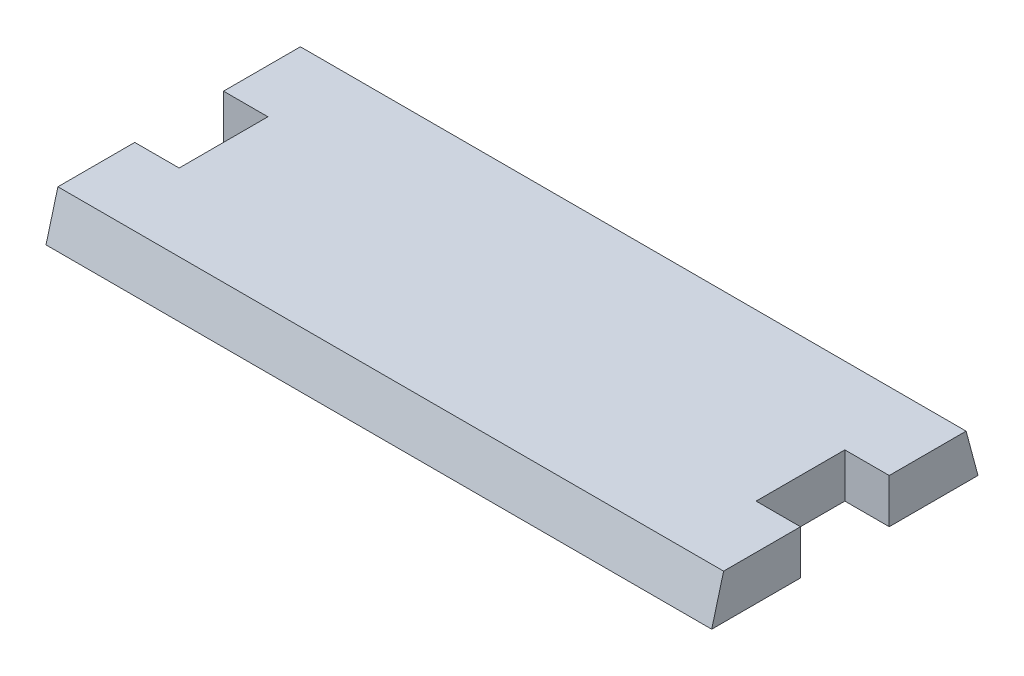
ISO-10303-21;
HEADER;
FILE_DESCRIPTION(('STEP AP214'),'2;1');
FILE_NAME('part.step','',(''),(''),'','','');
FILE_SCHEMA(('AUTOMOTIVE_DESIGN { 1 0 10303 214 1 1 1 1 }'));
ENDSEC;
DATA;
#1=APPLICATION_CONTEXT('core data for automotive mechanical design processes');
#2=APPLICATION_PROTOCOL_DEFINITION('international standard','automotive_design',2000,#1);
#3=PRODUCT_CONTEXT('',#1,'mechanical');
#4=PRODUCT('Part','Part','',(#3));
#5=PRODUCT_RELATED_PRODUCT_CATEGORY('part','',(#4));
#6=PRODUCT_DEFINITION_FORMATION('','',#4);
#7=PRODUCT_DEFINITION_CONTEXT('part definition',#1,'design');
#8=PRODUCT_DEFINITION('design','',#6,#7);
#9=PRODUCT_DEFINITION_SHAPE('','',#8);
#10=(LENGTH_UNIT() NAMED_UNIT(*) SI_UNIT(.MILLI.,.METRE.));
#11=(NAMED_UNIT(*) PLANE_ANGLE_UNIT() SI_UNIT($,.RADIAN.));
#12=(NAMED_UNIT(*) SI_UNIT($,.STERADIAN.) SOLID_ANGLE_UNIT());
#13=UNCERTAINTY_MEASURE_WITH_UNIT(LENGTH_MEASURE(1.E-05),#10,'distance_accuracy_value','');
#14=(GEOMETRIC_REPRESENTATION_CONTEXT(3) GLOBAL_UNCERTAINTY_ASSIGNED_CONTEXT((#13)) GLOBAL_UNIT_ASSIGNED_CONTEXT((#10,
#11,#12)) REPRESENTATION_CONTEXT('',''));
#15=CARTESIAN_POINT('',(0.,0.,0.));
#16=DIRECTION('',(0.,0.,1.));
#17=DIRECTION('',(1.,0.,0.));
#18=AXIS2_PLACEMENT_3D('',#15,#16,#17);
#19=CARTESIAN_POINT('',(0.,5.,0.));
#20=DIRECTION('',(1.,0.,0.));
#21=DIRECTION('',(0.,0.,-1.));
#22=AXIS2_PLACEMENT_3D('',#19,#20,#21);
#23=PLANE('',#22);
#24=DIRECTION('',(0.,0.,1.));
#25=VECTOR('',#24,1.);
#26=CARTESIAN_POINT('',(0.,-5.,0.));
#27=LINE('',#26,#25);
#28=CARTESIAN_POINT('',(0.,-5.,-20.));
#29=VERTEX_POINT('',#28);
#30=CARTESIAN_POINT('',(0.,-5.,0.));
#31=VERTEX_POINT('',#30);
#32=EDGE_CURVE('E160',#29,#31,#27,.T.);
#33=ORIENTED_EDGE('',*,*,#32,.T.);
#34=DIRECTION('',(0.,0.965925826289068,-0.258819045102521));
#35=VECTOR('',#34,1.);
#36=CARTESIAN_POINT('',(0.,-5.,0.));
#37=LINE('',#36,#35);
#38=CARTESIAN_POINT('',(0.,5.,-2.67949192431123));
#39=VERTEX_POINT('',#38);
#40=EDGE_CURVE('E11',#39,#31,#37,.F.);
#41=ORIENTED_EDGE('',*,*,#40,.F.);
#42=DIRECTION('',(0.,0.,1.));
#43=VECTOR('',#42,1.);
#44=CARTESIAN_POINT('',(0.,5.,0.));
#45=LINE('',#44,#43);
#46=CARTESIAN_POINT('',(0.,5.,-20.));
#47=VERTEX_POINT('',#46);
#48=EDGE_CURVE('E182',#47,#39,#45,.T.);
#49=ORIENTED_EDGE('',*,*,#48,.F.);
#50=DIRECTION('',(0.,-1.,0.));
#51=VECTOR('',#50,1.);
#52=CARTESIAN_POINT('',(0.,5.,-20.));
#53=LINE('',#52,#51);
#54=EDGE_CURVE('E153',#47,#29,#53,.T.);
#55=ORIENTED_EDGE('',*,*,#54,.T.);
#56=EDGE_LOOP('',(#33,#41,#49,#55));
#57=FACE_BOUND('',#56,.T.);
#58=ADVANCED_FACE('F39',(#57),#23,.F.);
#59=CARTESIAN_POINT('',(0.,-5.,0.));
#60=DIRECTION('',(0.,0.258819045102521,0.965925826289068));
#61=DIRECTION('',(0.,-0.965925826289068,0.258819045102521));
#62=AXIS2_PLACEMENT_3D('',#59,#60,#61);
#63=PLANE('',#62);
#64=DIRECTION('',(1.,0.,0.));
#65=VECTOR('',#64,1.);
#66=CARTESIAN_POINT('',(0.,-5.,0.));
#67=LINE('',#66,#65);
#68=CARTESIAN_POINT('',(150.,-5.,0.));
#69=VERTEX_POINT('',#68);
#70=EDGE_CURVE('E159',#31,#69,#67,.T.);
#71=ORIENTED_EDGE('',*,*,#70,.T.);
#72=DIRECTION('',(0.,0.965925826289068,-0.258819045102521));
#73=VECTOR('',#72,1.);
#74=CARTESIAN_POINT('',(150.,4.33012701892219,-2.50000000000001));
#75=LINE('',#74,#73);
#76=CARTESIAN_POINT('',(150.,5.,-2.67949192431123));
#77=VERTEX_POINT('',#76);
#78=EDGE_CURVE('E47',#77,#69,#75,.F.);
#79=ORIENTED_EDGE('',*,*,#78,.F.);
#80=DIRECTION('',(-1.,0.,0.));
#81=VECTOR('',#80,1.);
#82=CARTESIAN_POINT('',(0.,5.,-2.67949192431123));
#83=LINE('',#82,#81);
#84=EDGE_CURVE('E200',#39,#77,#83,.F.);
#85=ORIENTED_EDGE('',*,*,#84,.F.);
#86=ORIENTED_EDGE('',*,*,#40,.T.);
#87=EDGE_LOOP('',(#71,#79,#85,#86));
#88=FACE_BOUND('',#87,.T.);
#89=ADVANCED_FACE('F221',(#88),#63,.T.);
#90=CARTESIAN_POINT('',(150.,5.,0.));
#91=DIRECTION('',(-1.,0.,0.));
#92=DIRECTION('',(0.,0.,1.));
#93=AXIS2_PLACEMENT_3D('',#90,#91,#92);
#94=PLANE('',#93);
#95=DIRECTION('',(0.,0.,-1.));
#96=VECTOR('',#95,1.);
#97=CARTESIAN_POINT('',(150.,-5.,0.));
#98=LINE('',#97,#96);
#99=CARTESIAN_POINT('',(150.,-5.,-20.));
#100=VERTEX_POINT('',#99);
#101=EDGE_CURVE('E165',#69,#100,#98,.T.);
#102=ORIENTED_EDGE('',*,*,#101,.T.);
#103=DIRECTION('',(0.,-1.,0.));
#104=VECTOR('',#103,1.);
#105=CARTESIAN_POINT('',(150.,5.,-20.));
#106=LINE('',#105,#104);
#107=CARTESIAN_POINT('',(150.,5.,-20.));
#108=VERTEX_POINT('',#107);
#109=EDGE_CURVE('E198',#108,#100,#106,.T.);
#110=ORIENTED_EDGE('',*,*,#109,.F.);
#111=DIRECTION('',(0.,0.,-1.));
#112=VECTOR('',#111,1.);
#113=CARTESIAN_POINT('',(150.,5.,0.));
#114=LINE('',#113,#112);
#115=EDGE_CURVE('E203',#77,#108,#114,.T.);
#116=ORIENTED_EDGE('',*,*,#115,.F.);
#117=ORIENTED_EDGE('',*,*,#78,.T.);
#118=EDGE_LOOP('',(#102,#110,#116,#117));
#119=FACE_BOUND('',#118,.T.);
#120=ADVANCED_FACE('F230',(#119),#94,.F.);
#121=CARTESIAN_POINT('',(140.,5.,-20.));
#122=DIRECTION('',(0.,0.,1.));
#123=DIRECTION('',(1.,0.,0.));
#124=AXIS2_PLACEMENT_3D('',#121,#122,#123);
#125=PLANE('',#124);
#126=DIRECTION('',(-1.,0.,0.));
#127=VECTOR('',#126,1.);
#128=CARTESIAN_POINT('',(140.,-5.,-20.));
#129=LINE('',#128,#127);
#130=CARTESIAN_POINT('',(140.,-5.,-20.));
#131=VERTEX_POINT('',#130);
#132=EDGE_CURVE('E163',#100,#131,#129,.T.);
#133=ORIENTED_EDGE('',*,*,#132,.T.);
#134=DIRECTION('',(0.,-1.,0.));
#135=VECTOR('',#134,1.);
#136=CARTESIAN_POINT('',(140.,5.,-20.));
#137=LINE('',#136,#135);
#138=CARTESIAN_POINT('',(140.,5.,-20.));
#139=VERTEX_POINT('',#138);
#140=EDGE_CURVE('E195',#139,#131,#137,.T.);
#141=ORIENTED_EDGE('',*,*,#140,.F.);
#142=DIRECTION('',(-1.,0.,0.));
#143=VECTOR('',#142,1.);
#144=CARTESIAN_POINT('',(140.,5.,-20.));
#145=LINE('',#144,#143);
#146=EDGE_CURVE('E213',#108,#139,#145,.T.);
#147=ORIENTED_EDGE('',*,*,#146,.F.);
#148=ORIENTED_EDGE('',*,*,#109,.T.);
#149=EDGE_LOOP('',(#133,#141,#147,#148));
#150=FACE_BOUND('',#149,.T.);
#151=ADVANCED_FACE('F237',(#150),#125,.F.);
#152=CARTESIAN_POINT('',(140.,5.,-40.));
#153=DIRECTION('',(-1.,0.,0.));
#154=DIRECTION('',(0.,0.,1.));
#155=AXIS2_PLACEMENT_3D('',#152,#153,#154);
#156=PLANE('',#155);
#157=DIRECTION('',(0.,0.,-1.));
#158=VECTOR('',#157,1.);
#159=CARTESIAN_POINT('',(140.,-5.,-40.));
#160=LINE('',#159,#158);
#161=CARTESIAN_POINT('',(140.,-5.,-40.));
#162=VERTEX_POINT('',#161);
#163=EDGE_CURVE('E167',#131,#162,#160,.T.);
#164=ORIENTED_EDGE('',*,*,#163,.T.);
#165=DIRECTION('',(0.,-1.,0.));
#166=VECTOR('',#165,1.);
#167=CARTESIAN_POINT('',(140.,5.,-40.));
#168=LINE('',#167,#166);
#169=CARTESIAN_POINT('',(140.,5.,-40.));
#170=VERTEX_POINT('',#169);
#171=EDGE_CURVE('E190',#170,#162,#168,.T.);
#172=ORIENTED_EDGE('',*,*,#171,.F.);
#173=DIRECTION('',(0.,0.,-1.));
#174=VECTOR('',#173,1.);
#175=CARTESIAN_POINT('',(140.,5.,-40.));
#176=LINE('',#175,#174);
#177=EDGE_CURVE('E207',#139,#170,#176,.T.);
#178=ORIENTED_EDGE('',*,*,#177,.F.);
#179=ORIENTED_EDGE('',*,*,#140,.T.);
#180=EDGE_LOOP('',(#164,#172,#178,#179));
#181=FACE_BOUND('',#180,.T.);
#182=ADVANCED_FACE('F238',(#181),#156,.F.);
#183=CARTESIAN_POINT('',(150.,5.,-40.));
#184=DIRECTION('',(0.,0.,-1.));
#185=DIRECTION('',(-1.,0.,0.));
#186=AXIS2_PLACEMENT_3D('',#183,#184,#185);
#187=PLANE('',#186);
#188=DIRECTION('',(1.,0.,0.));
#189=VECTOR('',#188,1.);
#190=CARTESIAN_POINT('',(150.,-5.,-40.));
#191=LINE('',#190,#189);
#192=CARTESIAN_POINT('',(150.,-5.,-40.));
#193=VERTEX_POINT('',#192);
#194=EDGE_CURVE('E169',#162,#193,#191,.T.);
#195=ORIENTED_EDGE('',*,*,#194,.T.);
#196=DIRECTION('',(0.,-1.,0.));
#197=VECTOR('',#196,1.);
#198=CARTESIAN_POINT('',(150.,5.,-40.));
#199=LINE('',#198,#197);
#200=CARTESIAN_POINT('',(150.,5.,-40.));
#201=VERTEX_POINT('',#200);
#202=EDGE_CURVE('E188',#201,#193,#199,.T.);
#203=ORIENTED_EDGE('',*,*,#202,.F.);
#204=DIRECTION('',(1.,0.,0.));
#205=VECTOR('',#204,1.);
#206=CARTESIAN_POINT('',(150.,5.,-40.));
#207=LINE('',#206,#205);
#208=EDGE_CURVE('E120',#170,#201,#207,.T.);
#209=ORIENTED_EDGE('',*,*,#208,.F.);
#210=ORIENTED_EDGE('',*,*,#171,.T.);
#211=EDGE_LOOP('',(#195,#203,#209,#210));
#212=FACE_BOUND('',#211,.T.);
#213=ADVANCED_FACE('F242',(#212),#187,.F.);
#214=CARTESIAN_POINT('',(150.,5.,-40.));
#215=DIRECTION('',(-1.,0.,0.));
#216=DIRECTION('',(0.,0.,1.));
#217=AXIS2_PLACEMENT_3D('',#214,#215,#216);
#218=PLANE('',#217);
#219=DIRECTION('',(0.,0.,-1.));
#220=VECTOR('',#219,1.);
#221=CARTESIAN_POINT('',(150.,-5.,-40.));
#222=LINE('',#221,#220);
#223=CARTESIAN_POINT('',(150.,-5.,-60.));
#224=VERTEX_POINT('',#223);
#225=EDGE_CURVE('E168',#193,#224,#222,.T.);
#226=ORIENTED_EDGE('',*,*,#225,.T.);
#227=DIRECTION('',(0.,0.965925826289068,0.258819045102521));
#228=VECTOR('',#227,1.);
#229=CARTESIAN_POINT('',(150.,-5.,-60.));
#230=LINE('',#229,#228);
#231=CARTESIAN_POINT('',(150.,5.,-57.3205080756888));
#232=VERTEX_POINT('',#231);
#233=EDGE_CURVE('E186',#232,#224,#230,.F.);
#234=ORIENTED_EDGE('',*,*,#233,.F.);
#235=DIRECTION('',(0.,0.,-1.));
#236=VECTOR('',#235,1.);
#237=CARTESIAN_POINT('',(150.,5.,-40.));
#238=LINE('',#237,#236);
#239=EDGE_CURVE('E115',#201,#232,#238,.T.);
#240=ORIENTED_EDGE('',*,*,#239,.F.);
#241=ORIENTED_EDGE('',*,*,#202,.T.);
#242=EDGE_LOOP('',(#226,#234,#240,#241));
#243=FACE_BOUND('',#242,.T.);
#244=ADVANCED_FACE('F249',(#243),#218,.F.);
#245=CARTESIAN_POINT('',(0.,-5.,-60.));
#246=DIRECTION('',(0.,0.258819045102521,-0.965925826289068));
#247=DIRECTION('',(0.,0.965925826289068,0.258819045102521));
#248=AXIS2_PLACEMENT_3D('',#245,#246,#247);
#249=PLANE('',#248);
#250=DIRECTION('',(-1.,0.,0.));
#251=VECTOR('',#250,1.);
#252=CARTESIAN_POINT('',(0.,-5.,-60.));
#253=LINE('',#252,#251);
#254=CARTESIAN_POINT('',(0.,-5.,-60.));
#255=VERTEX_POINT('',#254);
#256=EDGE_CURVE('E174',#224,#255,#253,.T.);
#257=ORIENTED_EDGE('',*,*,#256,.T.);
#258=DIRECTION('',(0.,0.965925826289068,0.258819045102521));
#259=VECTOR('',#258,1.);
#260=CARTESIAN_POINT('',(0.,9.3301270189222,-56.1602540378444));
#261=LINE('',#260,#259);
#262=CARTESIAN_POINT('',(0.,5.,-57.3205080756888));
#263=VERTEX_POINT('',#262);
#264=EDGE_CURVE('E43',#263,#255,#261,.F.);
#265=ORIENTED_EDGE('',*,*,#264,.F.);
#266=DIRECTION('',(1.,0.,0.));
#267=VECTOR('',#266,1.);
#268=CARTESIAN_POINT('',(0.,5.,-57.3205080756888));
#269=LINE('',#268,#267);
#270=EDGE_CURVE('E202',#232,#263,#269,.F.);
#271=ORIENTED_EDGE('',*,*,#270,.F.);
#272=ORIENTED_EDGE('',*,*,#233,.T.);
#273=EDGE_LOOP('',(#257,#265,#271,#272));
#274=FACE_BOUND('',#273,.T.);
#275=ADVANCED_FACE('F41',(#274),#249,.T.);
#276=CARTESIAN_POINT('',(0.,5.,-40.));
#277=DIRECTION('',(1.,0.,0.));
#278=DIRECTION('',(0.,0.,-1.));
#279=AXIS2_PLACEMENT_3D('',#276,#277,#278);
#280=PLANE('',#279);
#281=DIRECTION('',(0.,0.,1.));
#282=VECTOR('',#281,1.);
#283=CARTESIAN_POINT('',(0.,-5.,-40.));
#284=LINE('',#283,#282);
#285=CARTESIAN_POINT('',(0.,-5.,-40.));
#286=VERTEX_POINT('',#285);
#287=EDGE_CURVE('E175',#255,#286,#284,.T.);
#288=ORIENTED_EDGE('',*,*,#287,.T.);
#289=DIRECTION('',(0.,-1.,0.));
#290=VECTOR('',#289,1.);
#291=CARTESIAN_POINT('',(0.,5.,-40.));
#292=LINE('',#291,#290);
#293=CARTESIAN_POINT('',(0.,5.,-40.));
#294=VERTEX_POINT('',#293);
#295=EDGE_CURVE('E150',#294,#286,#292,.T.);
#296=ORIENTED_EDGE('',*,*,#295,.F.);
#297=DIRECTION('',(0.,0.,1.));
#298=VECTOR('',#297,1.);
#299=CARTESIAN_POINT('',(0.,5.,-40.));
#300=LINE('',#299,#298);
#301=EDGE_CURVE('E131',#263,#294,#300,.T.);
#302=ORIENTED_EDGE('',*,*,#301,.F.);
#303=ORIENTED_EDGE('',*,*,#264,.T.);
#304=EDGE_LOOP('',(#288,#296,#302,#303));
#305=FACE_BOUND('',#304,.T.);
#306=ADVANCED_FACE('F252',(#305),#280,.F.);
#307=CARTESIAN_POINT('',(0.,5.,-40.));
#308=DIRECTION('',(0.,0.,-1.));
#309=DIRECTION('',(-1.,0.,0.));
#310=AXIS2_PLACEMENT_3D('',#307,#308,#309);
#311=PLANE('',#310);
#312=DIRECTION('',(1.,0.,0.));
#313=VECTOR('',#312,1.);
#314=CARTESIAN_POINT('',(0.,-5.,-40.));
#315=LINE('',#314,#313);
#316=CARTESIAN_POINT('',(10.,-5.,-40.));
#317=VERTEX_POINT('',#316);
#318=EDGE_CURVE('E145',#286,#317,#315,.T.);
#319=ORIENTED_EDGE('',*,*,#318,.T.);
#320=DIRECTION('',(0.,-1.,0.));
#321=VECTOR('',#320,1.);
#322=CARTESIAN_POINT('',(10.,5.,-40.));
#323=LINE('',#322,#321);
#324=CARTESIAN_POINT('',(10.,5.,-40.));
#325=VERTEX_POINT('',#324);
#326=EDGE_CURVE('E143',#325,#317,#323,.T.);
#327=ORIENTED_EDGE('',*,*,#326,.F.);
#328=DIRECTION('',(1.,0.,0.));
#329=VECTOR('',#328,1.);
#330=CARTESIAN_POINT('',(0.,5.,-40.));
#331=LINE('',#330,#329);
#332=EDGE_CURVE('E126',#294,#325,#331,.T.);
#333=ORIENTED_EDGE('',*,*,#332,.F.);
#334=ORIENTED_EDGE('',*,*,#295,.T.);
#335=EDGE_LOOP('',(#319,#327,#333,#334));
#336=FACE_BOUND('',#335,.T.);
#337=ADVANCED_FACE('F142',(#336),#311,.F.);
#338=CARTESIAN_POINT('',(10.,5.,-40.));
#339=DIRECTION('',(1.,0.,0.));
#340=DIRECTION('',(0.,0.,-1.));
#341=AXIS2_PLACEMENT_3D('',#338,#339,#340);
#342=PLANE('',#341);
#343=DIRECTION('',(0.,0.,1.));
#344=VECTOR('',#343,1.);
#345=CARTESIAN_POINT('',(10.,-5.,-40.));
#346=LINE('',#345,#344);
#347=CARTESIAN_POINT('',(10.,-5.,-20.));
#348=VERTEX_POINT('',#347);
#349=EDGE_CURVE('E176',#317,#348,#346,.T.);
#350=ORIENTED_EDGE('',*,*,#349,.T.);
#351=DIRECTION('',(0.,-1.,0.));
#352=VECTOR('',#351,1.);
#353=CARTESIAN_POINT('',(10.,5.,-20.));
#354=LINE('',#353,#352);
#355=CARTESIAN_POINT('',(10.,5.,-20.));
#356=VERTEX_POINT('',#355);
#357=EDGE_CURVE('E146',#356,#348,#354,.T.);
#358=ORIENTED_EDGE('',*,*,#357,.F.);
#359=DIRECTION('',(0.,0.,1.));
#360=VECTOR('',#359,1.);
#361=CARTESIAN_POINT('',(10.,5.,-40.));
#362=LINE('',#361,#360);
#363=EDGE_CURVE('E134',#325,#356,#362,.T.);
#364=ORIENTED_EDGE('',*,*,#363,.F.);
#365=ORIENTED_EDGE('',*,*,#326,.T.);
#366=EDGE_LOOP('',(#350,#358,#364,#365));
#367=FACE_BOUND('',#366,.T.);
#368=ADVANCED_FACE('F147',(#367),#342,.F.);
#369=CARTESIAN_POINT('',(10.,5.,-20.));
#370=DIRECTION('',(0.,0.,1.));
#371=DIRECTION('',(1.,0.,0.));
#372=AXIS2_PLACEMENT_3D('',#369,#370,#371);
#373=PLANE('',#372);
#374=DIRECTION('',(-1.,0.,0.));
#375=VECTOR('',#374,1.);
#376=CARTESIAN_POINT('',(10.,-5.,-20.));
#377=LINE('',#376,#375);
#378=EDGE_CURVE('E178',#348,#29,#377,.T.);
#379=ORIENTED_EDGE('',*,*,#378,.T.);
#380=ORIENTED_EDGE('',*,*,#54,.F.);
#381=DIRECTION('',(-1.,0.,0.));
#382=VECTOR('',#381,1.);
#383=CARTESIAN_POINT('',(10.,5.,-20.));
#384=LINE('',#383,#382);
#385=EDGE_CURVE('E59',#356,#47,#384,.T.);
#386=ORIENTED_EDGE('',*,*,#385,.F.);
#387=ORIENTED_EDGE('',*,*,#357,.T.);
#388=EDGE_LOOP('',(#379,#380,#386,#387));
#389=FACE_BOUND('',#388,.T.);
#390=ADVANCED_FACE('F260',(#389),#373,.F.);
#391=CARTESIAN_POINT('',(0.,5.,0.));
#392=DIRECTION('',(0.,1.,0.));
#393=DIRECTION('',(0.,0.,1.));
#394=AXIS2_PLACEMENT_3D('',#391,#392,#393);
#395=PLANE('',#394);
#396=ORIENTED_EDGE('',*,*,#48,.T.);
#397=ORIENTED_EDGE('',*,*,#84,.T.);
#398=ORIENTED_EDGE('',*,*,#115,.T.);
#399=ORIENTED_EDGE('',*,*,#146,.T.);
#400=ORIENTED_EDGE('',*,*,#177,.T.);
#401=ORIENTED_EDGE('',*,*,#208,.T.);
#402=ORIENTED_EDGE('',*,*,#239,.T.);
#403=ORIENTED_EDGE('',*,*,#270,.T.);
#404=ORIENTED_EDGE('',*,*,#301,.T.);
#405=ORIENTED_EDGE('',*,*,#332,.T.);
#406=ORIENTED_EDGE('',*,*,#363,.T.);
#407=ORIENTED_EDGE('',*,*,#385,.T.);
#408=EDGE_LOOP('',(#396,#397,#398,#399,#400,#401,#402,#403,#404,#405,#406,#407));
#409=FACE_BOUND('',#408,.T.);
#410=ADVANCED_FACE('F128',(#409),#395,.T.);
#411=CARTESIAN_POINT('',(0.,-5.,0.));
#412=DIRECTION('',(0.,1.,0.));
#413=DIRECTION('',(0.,0.,1.));
#414=AXIS2_PLACEMENT_3D('',#411,#412,#413);
#415=PLANE('',#414);
#416=ORIENTED_EDGE('',*,*,#32,.F.);
#417=ORIENTED_EDGE('',*,*,#378,.F.);
#418=ORIENTED_EDGE('',*,*,#349,.F.);
#419=ORIENTED_EDGE('',*,*,#318,.F.);
#420=ORIENTED_EDGE('',*,*,#287,.F.);
#421=ORIENTED_EDGE('',*,*,#256,.F.);
#422=ORIENTED_EDGE('',*,*,#225,.F.);
#423=ORIENTED_EDGE('',*,*,#194,.F.);
#424=ORIENTED_EDGE('',*,*,#163,.F.);
#425=ORIENTED_EDGE('',*,*,#132,.F.);
#426=ORIENTED_EDGE('',*,*,#101,.F.);
#427=ORIENTED_EDGE('',*,*,#70,.F.);
#428=EDGE_LOOP('',(#416,#417,#418,#419,#420,#421,#422,#423,#424,#425,#426,#427));
#429=FACE_BOUND('',#428,.T.);
#430=ADVANCED_FACE('F255',(#429),#415,.F.);
#431=CLOSED_SHELL('',(#58,#89,#120,#151,#182,#213,#244,#275,#306,#337,#368,#390,#410,#430));
#432=MANIFOLD_SOLID_BREP('B2',#431);
#433=ADVANCED_BREP_SHAPE_REPRESENTATION('',(#18,#432),#14);
#434=SHAPE_DEFINITION_REPRESENTATION(#9,#433);
ENDSEC;
END-ISO-10303-21;
